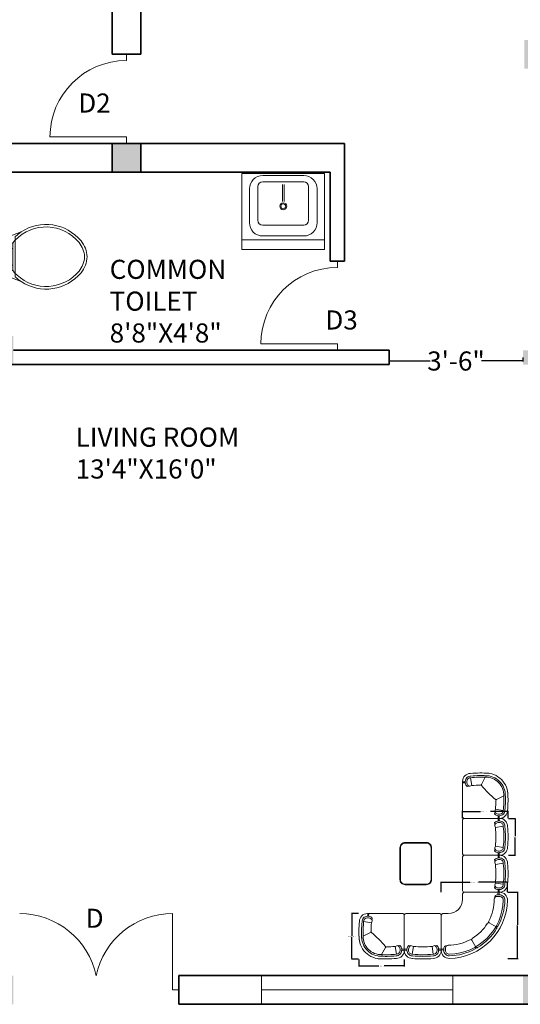
# Model space of a CAD drawing. Units: inches. Extents: x -36302355 to 648, y -221479757 to 75.
# Tile 13 of 37: x 285 to 442, y -580 to -271. Entities that reach past the tile are written whole.
import ezdxf

# ---------------------------------------------------------------- set-up
doc = ezdxf.new("R2010")
doc.units = ezdxf.units.IN
doc.header["$MEASUREMENT"] = 0
for name, color, linetype, lineweight in [('A-ANNO-DIMS', 2, 'Continuous', 18), ('A-ANNO-IDEN', 7, 'Continuous', 18), ('A-AREA-IDEN', 7, 'Continuous', 18), ('A-COLS', 7, 'Continuous', 35), ('A-COLS-PATT', 242, 'Continuous', 13), ('A-DOOR', 4, 'Continuous', 18), ('A-FLOR-FIXT', 9, 'Continuous', 18), ('A-FURN', 8, 'Continuous', 13), ('A-GLAZ', 142, 'Continuous', 18), ('A-WALL', 7, 'Continuous', 35)]:
    doc.layers.add(name, color=color, linetype=linetype, lineweight=lineweight)
doc.styles.get("Standard").update_dxf_attribs({"font": 'arial.ttf'})
doc.dimstyles.get("Standard").update_dxf_attribs({"dimtxt": 0.18, "dimasz": 0.18, "dimexe": 0.18, "dimexo": 0.0625, "dimgap": 0.09, "dimtad": 0, "dimtih": 1, "dimtoh": 1, "dimdec": 0, "dimzin": 0, "dimdsep": 46, "dimlunit": 3, "dimtxsty": 'Standard', "dimcen": 0.09, "dimadec": 0, "dimazin": 0, "dimtfac": 1, "dimtdec": 0, "dimtofl": 0, "dimtmove": 0, "dimatfit": 3, "dimfxl": 1, "dimtolj": 1, "dimtzin": 0, "dimarcsym": 0})

# ---------------------------------------------------------------- blocks, each defined once
blk = doc.blocks.new('*D5')
at = {"layer": 'A-ANNO-DIMS', "color": 0, "lineweight": -2, "transparency": 16777216}
for p, q in [((401.2, -376.83), (401.2, -378.08)), ((443.2, -376.83), (443.2, -378.08)), ((401.38, -377.9), (414.13, -377.9)), ((443.02, -377.9), (430.26, -377.9))]:
    blk.add_line(p, q, dxfattribs=at)
at = {"layer": 'A-ANNO-DIMS', "color": 0, "transparency": 16777216}
for points in [[(401.38, -377.87), (401.38, -377.93), (401.2, -377.9)], [(443.02, -377.87), (443.02, -377.93), (443.2, -377.9)]]:
    blk.add_solid(points, dxfattribs=at)
at = {"layer": 'Defpoints', "color": 0, "transparency": 16777216}
for p in [(401.2, -376.77), (443.2, -376.77), (443.2, -377.9)]:
    blk.add_point(p, dxfattribs=at)
at = {"layer": 'A-ANNO-DIMS', "color": 0, "transparency": 16777216, "insert": (422.2, -377.9), "char_height": 6, "attachment_point": 5}
blk.add_mtext('\\A1;3\'-6"', dxfattribs=at)
blk = doc.blocks.new('A$C707258B2')
at = {"color": 0}
for p, q in [((0.404, 0.342), (1.074, 0.342)), ((0.404, 0.292), (0.454, 0.292)), ((0.404, 0.262), (0.454, 0.262)), ((1.104, 0.312), (1.104, 0.212)), ((1.479, -0.063), (1.379, -0.063)), ((1.509, -0.763), (1.509, -0.093)), ((0.6, -0.238), (0.47, -0.313)), ((0.929, -0.567), (0.854, -0.697)), ((1.429, -0.763), (1.429, -0.713)), ((1.459, -0.763), (1.459, -0.712))]:
    blk.add_line(p, q, dxfattribs=at)
for centre, radius, start, end in [((0.404, 0.192), 0.15, 90, 181.1754), ((1.379, 0.212), 1.125, 181.1754, 268.8246), ((0.404, 0.192), 0.1, 90, 181.1754), ((1.379, 0.212), 1.075, 181.1754, 208.6357), ((0.404, 0.192), 0.07, 90, 181.1754), ((1.379, 0.212), 1.045, 181.1754, 268.8246), ((0.378, 0.317), 0.0362, 316.3972, 43.6028), ((0.368, 0.317), 0.0662, 337.8298, 22.1702), ((0.455, 0.256), 0.0357, 345.4262, 90.5555), ((0.454, 0.212), 0.05, 360, 90), ((1.379, 0.212), 0.875, 180, 208.4082), ((1.074, 0.312), 0.03, 360, 90), ((1.379, 0.212), 0.275, 180, 270), ((1.479, -0.093), 0.03, 360, 90), ((0.457, -0.291), 0.025, 208.6357, 300), ((0.482, -0.334), 0.025, 120, 211.3643), ((1.379, 0.212), 1.075, 211.3643, 238.6357), ((0.587, -0.216), 0.025, 300, 28.4082), ((0.612, -0.259), 0.025, 31.5918, 120), ((1.379, 0.212), 0.875, 211.5918, 238.4082), ((0.907, -0.555), 0.025, 330, 58.4082), ((0.951, -0.58), 0.025, 61.5918, 150), ((1.379, 0.212), 0.875, 241.5918, 270), ((0.832, -0.685), 0.025, 238.6357, 330), ((0.876, -0.71), 0.025, 150, 241.3643), ((1.379, 0.212), 1.075, 241.3643, 268.8246), ((1.379, -0.713), 0.05, 360, 90), ((1.425, -0.709), 0.0336, 354.6301, 109.3883), ((1.484, -0.799), 0.0662, 67.8298, 112.1702), ((1.359, -0.763), 0.15, 268.8246, 360), ((1.359, -0.763), 0.1, 268.8246, 360), ((1.359, -0.763), 0.07, 268.8246, 360), ((1.484, -0.789), 0.0362, 46.3972, 133.6028)]:
    blk.add_arc(centre, radius, start, end, dxfattribs=at)
blk = doc.blocks.new('part 01')
at = {"color": 0}
for p, q in [((-670, 700), (0, 700)), ((-591, 527), (-579, 561)), ((30, 30), (30, 670)), ((-591, 527), (-740, 550)), ((-591, 173), (-740, 150)), ((-670, 0), (0, 0)), ((-591, 173), (-579, 139))]:
    blk.add_line(p, q, dxfattribs=at)
for centre, radius, start, end in [((-670, 550), 150, 90, 181.1754), ((-670, 550), 100, 90, 181.1754), ((-670, 550), 70, 90, 181.1754), ((-660, 518), 133, 56.0897, 95.6132), ((-696, 675), 36.2, 316.3972, 43.6028), ((-660, 518), 103, 42.0066, 95.6132), ((-706, 675), 66.2, 337.8298, 22.1702), ((-600, 607), 25, 332.9608, 56.0897), ((-625, 620), 53.2, 321.0017, 332.9608), ((-602, 570), 25, 340, 42.0066), ((0, 670), 30, 0, 90), ((1178, 350), 2008, 174.2835, 185.7165), ((1178, 350), 1958, 174.2835, 185.7165), ((1178, 350), 1928, 174.2835, 185.7165), ((1178, 350), 1778, 174.2835, 185.7165), ((-670, 150), 150, 178.8246, 270), ((-670, 150), 100, 178.8246, 270), ((-670, 150), 70, 178.8246, 270), ((-660, 182), 133, 264.3868, 303.9103), ((-660, 182), 103, 264.3868, 317.9934), ((-696, 25), 36.2, 316.3972, 43.6028), ((-706, 25), 66.2, 337.8298, 22.1702), ((-600, 93), 25, 303.9103, 27.0392), ((-602, 130), 25, 317.9934, 20), ((-625, 80), 53.2, 27.0392, 38.9983), ((0, 30), 30, 270, 0)]:
    blk.add_arc(centre, radius, start, end, dxfattribs=at)
blk = doc.blocks.new('part02')
at = {"color": 0}
for p, q in [((0, -670), (0, 0)), ((30, 30), (700, 30)), ((621, -143), (609, -109)), ((621, -143), (770, -120)), ((640, -326), (778, -399)), ((173, -591), (139, -579)), ((173, -591), (150, -740)), ((356, -610), (429, -748))]:
    blk.add_line(p, q, dxfattribs=at)
for centre, radius, start, end in [((30, 0), 30, 90, 180), ((726, 5), 56.2, 153.6122, 206.6666), ((726, 5), 36.2, 136.3972, 223.6028), ((700, -120), 150, 0, 90), ((630, -63), 25, 123.9103, 207.0392), ((655, -50), 53.2, 207.0392, 218.9983), ((632, -100), 25, 137.9934, 200), ((690, -152), 103, 84.3868, 137.9934), ((689, -151), 132, 85.4378, 123.9887), ((-1148, -320), 1778, 0.3836, 5.7165), ((700, -121), 101, 357.5006, 89.858), ((700, -120), 70, 0, 90), ((-1228, -320), 2008, 357.7349, 5.7032), ((-1148, -320), 1958, 355.8657, 5.7165), ((-1148, -320), 2008, 355.818, 5.7165), ((2220, -2190), 2454, 130.6961, 139.3039), ((632, -344), 20, 62, 130.6961), ((650, -308), 20, 180.3836, 242), ((439, -409), 419, 268.2181, 1.7819), ((439, -409), 369, 268.2181, 1.7819), ((439, -409), 339, 268.2181, 1.7819), ((25, -696), 56.2, 63.3334, 116.3878), ((25, -696), 36.2, 46.3972, 133.6028), ((150, -670), 150, 180, 271.1754), ((182, -660), 133, 146.0897, 185.6132), ((150, -670), 100, 180, 271.1754), ((93, -600), 25, 62.9608, 146.0897), ((182, -660), 103, 132.0066, 185.6132), ((150, -670), 70, 180, 270), ((80, -625), 53.2, 51.0017, 62.9608), ((130, -602), 25, 70, 132.0066), ((350, 1258), 2008, 264.2968, 272.2651), ((350, 1178), 1778, 264.2835, 269.6164), ((338, -620), 20, 28, 89.6164), ((374, -602), 20, 139.3039, 208), ((350, 1178), 2008, 264.2835, 274.182), ((350, 1178), 1958, 264.2835, 274.1343)]:
    blk.add_arc(centre, radius, start, end, dxfattribs=at)
blk = doc.blocks.new('М14 600х655')
for p, q in [((-655, 600), (-655, 0)), ((-655, 600), (-655, 0)), ((-655, 0), (-655, 600)), ((0, 600), (-655, 600)), ((0, 0), (0, 600)), ((0, 525), (-655, 525)), ((-165.1, 494.1), (-489.9, 494.1)), ((-165.4, 408.4), (-490.2, 408.4)), ((-595.8, 388.1), (-595.8, 121.3)), ((-528.4, 370.1), (-528.4, 103.3)), ((-127.2, 103.3), (-127.2, 370.1)), ((-59.2, 121.3), (-59.2, 388.1)), ((-333.5, 87.1), (-333.5, 219.6)), ((-321.5, 87.1), (-321.5, 219.6)), ((-655, 0), (-655, 0)), ((-655, 0), (-655, 0)), ((-655, 0), (0, 0)), ((-655, 0), (0, 0)), ((-490.2, 65.1), (-165.4, 65.1)), ((-489.9, 15.4), (-165.1, 15.4))]:
    blk.add_line(p, q)
for radius in [27.6, 19.3]:
    blk.add_circle((-327.5, 258.9), radius)
for centre, radius, start, end in [((-489.9, 388.1), 105.9, 90, 180), ((-165.1, 388.1), 105.9, 0, 90), ((-490.2, 370.1), 38.2, 90, 180), ((-165.4, 370.1), 38.2, 0, 90), ((-489.9, 121.3), 105.9, 180, 270), ((-490.2, 103.3), 38.2, 180, 270), ((-165.4, 103.3), 38.2, 270, 0), ((-165.1, 121.3), 105.9, 270, 0)]:
    blk.add_arc(centre, radius, start, end)
blk = doc.blocks.new('WC-FLOOR-MOUNT')
for p, q in [((4.02, 15.38), (4.02, 16.49)), ((4.02, 15.38), (4.02, 10.15)), ((4.02, 4.92), (4.02, 10.15)), ((4.02, 3.8), (4.02, 4.92))]:
    blk.add_line(p, q)
for points in [[(4.02, 15.38, -0.448546), (24.05, 14.64, -0.162618), (25.78, 10.15, -0.470877)], [(5.85, 17.93, -0.383919), (24.66, 15.14, -0.163732), (26.58, 10.15, -0.359733)], [(0, 10.15), (0, 15.22, -0.31031), (0.43, 15.85), (5.85, 17.93, -0.209071)], [(4.02, 16.49, -0.040937), (5.85, 17.93, -0.163732)], [(3.22, 14.46), (2.11, 14.46, 1), (2.11, 12.77), (2.69, 12.77)], [(3.22, 14.46, -0.022712), (4.02, 15.38, -0.162618)], [(3.22, 10.15), (3.22, 14.46, -0.476108)], [(0, 10.15), (0, 5.07, 0.31031), (0.43, 4.45), (5.85, 2.37, 0.209071)], [(3.22, 10.15), (3.22, 5.84, 0.022712)], [(4.57, 4.39, 0.431639), (24.05, 5.66, 0.162618), (25.78, 10.15, 0.470877)], [(5.85, 2.37, 0.383919), (24.66, 5.15, 0.163732), (26.58, 10.15, 0.359733)], [(3.22, 5.84), (2.11, 5.84, -1), (2.11, 7.53), (2.69, 7.53)], [(3.22, 5.84, 0.022712), (4.02, 4.92, 0.162618)], [(4.02, 4.92, 0.014165), (4.57, 4.39, 0.162618)], [(4.02, 3.8, 0.040937), (5.85, 2.37, 0.163732)]]:
    blk.add_lwpolyline(points, format="xyb")
for points in [[(2.69, 12.77), (2.69, 7.53)], [(2.69, 12.77), (3.22, 12.77)], [(2.69, 7.53), (3.22, 7.53)]]:
    blk.add_lwpolyline(points)
blk = doc.blocks.new('WIN-60')
for p, q in [((60, 9), (0, 9)), ((0, 9), (0, 0)), ((60, 0), (60, 9)), ((0, 4.5), (60, 4.5)), ((0, 0), (60, 0))]:
    blk.add_line(p, q)
blk = doc.blocks.new('DOOR-SWING-24')
for p, q in [((0, 26), (0, 28)), ((0, 0), (0, 2)), ((0, 2), (24, 2))]:
    blk.add_line(p, q)
blk.add_arc((0, 2), 24, 0, 90)
blk = doc.blocks.new('*D35')
at = {"layer": 'A-ANNO-DIMS', "color": 0, "lineweight": -2, "transparency": 16777216}
for p, q in [((424.29, -521.53), (424.29, -519.27)), ((424.47, -519.45), (429.85, -519.45)), ((438.42, -519.45), (433.03, -519.45)), ((438.6, -521.53), (438.6, -519.27))]:
    blk.add_line(p, q, dxfattribs=at)
at = {"layer": 'A-ANNO-DIMS', "color": 0, "transparency": 16777216}
for points in [[(424.47, -519.42), (424.47, -519.48), (424.29, -519.45)], [(438.42, -519.42), (438.42, -519.48), (438.6, -519.45)]]:
    blk.add_solid(points, dxfattribs=at)
at = {"layer": 'Defpoints', "color": 0, "transparency": 16777216}
for p in [(424.29, -519.45), (424.29, -521.59), (438.6, -521.59)]:
    blk.add_point(p, dxfattribs=at)
at = {"layer": 'A-ANNO-DIMS', "color": 0, "transparency": 16777216, "insert": (431.44, -519.45), "char_height": 0.18, "attachment_point": 5}
blk.add_mtext('\\A1;SOFA SEAT 1\'-2 1/2" TYP.', dxfattribs=at)
blk = doc.blocks.new('*D36')
at = {"layer": 'A-ANNO-DIMS', "color": 0, "lineweight": -2, "transparency": 16777216}
for p, q in [((438.66, -521.59), (440.92, -521.59)), ((440.74, -521.77), (440.74, -527.21)), ((440.74, -533.02), (440.74, -527.58)), ((438.66, -533.2), (440.92, -533.2))]:
    blk.add_line(p, q, dxfattribs=at)
at = {"layer": 'A-ANNO-DIMS', "color": 0, "transparency": 16777216}
for points in [[(440.71, -521.77), (440.77, -521.77), (440.74, -521.59)], [(440.71, -533.02), (440.77, -533.02), (440.74, -533.2)]]:
    blk.add_solid(points, dxfattribs=at)
at = {"layer": 'Defpoints', "color": 0, "transparency": 16777216}
for p in [(438.6, -521.59), (440.74, -521.59), (438.6, -533.2)]:
    blk.add_point(p, dxfattribs=at)
at = {"layer": 'A-ANNO-DIMS', "color": 0, "transparency": 16777216, "insert": (440.74, -527.4), "char_height": 0.18, "attachment_point": 5}
blk.add_mtext('\\A1;0\'-11 1/2" TYP.', dxfattribs=at)
blk = doc.blocks.new('*D51')
at = {"layer": 'A-ANNO-DIMS', "color": 0, "lineweight": -2, "transparency": 16777216}
for p, q in [((391.6, -551.52), (389.34, -551.52)), ((389.52, -551.7), (389.52, -558.49)), ((389.52, -565.64), (389.52, -558.85)), ((391.6, -565.82), (389.34, -565.82))]:
    blk.add_line(p, q, dxfattribs=at)
at = {"layer": 'A-ANNO-DIMS', "color": 0, "transparency": 16777216}
for points in [[(389.49, -551.7), (389.55, -551.7), (389.52, -551.52)], [(389.49, -565.64), (389.55, -565.64), (389.52, -565.82)]]:
    blk.add_solid(points, dxfattribs=at)
at = {"layer": 'Defpoints', "color": 0, "transparency": 16777216}
for p in [(389.52, -551.52), (391.66, -551.52), (391.66, -565.82)]:
    blk.add_point(p, dxfattribs=at)
at = {"layer": 'A-ANNO-DIMS', "color": 0, "transparency": 16777216, "insert": (389.52, -558.67), "char_height": 0.18, "attachment_point": 5}
blk.add_mtext('\\A1;SOFA END 1\'-2 1/2" TYP.', dxfattribs=at)
blk = doc.blocks.new('*D52')
at = {"layer": 'A-ANNO-DIMS', "color": 0, "lineweight": -2, "transparency": 16777216}
for p, q in [((391.66, -565.89), (391.66, -568.15)), ((405.97, -565.89), (405.97, -568.15)), ((391.84, -567.97), (397.98, -567.97)), ((405.79, -567.97), (399.66, -567.97))]:
    blk.add_line(p, q, dxfattribs=at)
at = {"layer": 'A-ANNO-DIMS', "color": 0, "transparency": 16777216}
for points in [[(391.84, -567.94), (391.84, -568), (391.66, -567.97)], [(405.79, -567.94), (405.79, -568), (405.97, -567.97)]]:
    blk.add_solid(points, dxfattribs=at)
at = {"layer": 'Defpoints', "color": 0, "transparency": 16777216}
for p in [(391.66, -565.82), (405.97, -565.82), (391.66, -567.97)]:
    blk.add_point(p, dxfattribs=at)
at = {"layer": 'A-ANNO-DIMS', "color": 0, "transparency": 16777216, "insert": (398.82, -567.97), "char_height": 0.18, "attachment_point": 5}
blk.add_mtext('\\A1;1\'-2 1/2" TYP.', dxfattribs=at)
blk = doc.blocks.new('*D55')
at = {"layer": 'A-ANNO-DIMS', "color": 0, "lineweight": -2, "transparency": 16777216}
for p, q in [((417.57, -544.74), (417.57, -541.5)), ((417.75, -541.68), (426.7, -541.68)), ((438.21, -541.68), (429.27, -541.68)), ((438.39, -544.74), (438.39, -541.5))]:
    blk.add_line(p, q, dxfattribs=at)
at = {"layer": 'A-ANNO-DIMS', "color": 0, "transparency": 16777216}
for points in [[(417.75, -541.65), (417.75, -541.71), (417.57, -541.68)], [(438.21, -541.65), (438.21, -541.71), (438.39, -541.68)]]:
    blk.add_solid(points, dxfattribs=at)
at = {"layer": 'Defpoints', "color": 0, "transparency": 16777216}
for p in [(417.57, -541.68), (417.57, -544.8), (438.39, -544.8)]:
    blk.add_point(p, dxfattribs=at)
at = {"layer": 'A-ANNO-DIMS', "color": 0, "transparency": 16777216, "insert": (427.98, -541.68), "char_height": 0.18, "attachment_point": 5}
blk.add_mtext('\\A1;SOFA CORNER 1\'-9"', dxfattribs=at)
blk = doc.blocks.new('*D56')
at = {"layer": 'A-ANNO-DIMS', "color": 0, "lineweight": -2, "transparency": 16777216}
for p, q in [((438.45, -544.8), (441.69, -544.8)), ((441.51, -544.98), (441.51, -555.03)), ((441.51, -565.44), (441.51, -555.39)), ((438.45, -565.62), (441.69, -565.62))]:
    blk.add_line(p, q, dxfattribs=at)
at = {"layer": 'A-ANNO-DIMS', "color": 0, "transparency": 16777216}
for points in [[(441.48, -544.98), (441.54, -544.98), (441.51, -544.8)], [(441.48, -565.44), (441.54, -565.44), (441.51, -565.62)]]:
    blk.add_solid(points, dxfattribs=at)
at = {"layer": 'Defpoints', "color": 0, "transparency": 16777216}
for p in [(438.39, -544.8), (441.51, -544.8), (438.39, -565.62)]:
    blk.add_point(p, dxfattribs=at)
at = {"layer": 'A-ANNO-DIMS', "color": 0, "transparency": 16777216, "insert": (441.51, -555.21), "char_height": 0.18, "attachment_point": 5}
blk.add_mtext('\\A1;1\'-9"', dxfattribs=at)

msp = doc.modelspace()

# ---------------------------------------------------------------- hatches: boundary and pattern name
at = {"layer": 'A-COLS-PATT'}
h = msp.add_hatch(color=256, dxfattribs=at)
h.dxf.hatch_style = 1
h.paths.add_polyline_path([(145.2, 24.98), (145.2, 15.98), (154.2, 15.98), (154.2, 24.98)])
h.paths.add_polyline_path([(247.2, 15.98), (247.2, 24.98), (238.2, 24.98), (238.2, 15.98)])
h.paths.add_polyline_path([(387.64, 15.98), (395.7, 15.98), (395.7, 24.98), (387.64, 24.98)])
h.paths.add_polyline_path([(451.26, 24.98), (443.7, 24.98), (443.7, 15.98), (451.26, 15.98)])
h.paths.add_polyline_path([(596.2, 15.98), (605.2, 15.98), (605.2, 24.98), (596.2, 24.98)])
h.paths.add_polyline_path([(238.2, -122.02), (238.2, -131.02), (247.2, -131.02), (247.2, -122.02)])
h.paths.add_polyline_path([(395.7, -122.02), (387.46, -122.02), (387.46, -131.02), (395.7, -131.02)])
h.paths.add_polyline_path([(448.2, -131.02), (453.73, -131.02), (453.73, -122.02), (443.7, -122.02), (443.7, -131.02)])
h.paths.add_polyline_path([(596.2, -131.02), (605.2, -131.02), (605.2, -122.02), (596.2, -122.02)])
h.paths.add_polyline_path([(145.2, -176.97), (154.2, -176.97), (154.2, -167.02), (145.2, -167.02)])
h.paths.add_polyline_path([(314.2, -176.97), (323.2, -176.97), (323.2, -167.02), (314.2, -167.02)])
h.paths.add_polyline_path([(154.2, -314.02), (154.2, -309.52), (145.2, -309.52), (145.2, -314.02)])
h.paths.add_polyline_path([(314.2, -309.52), (314.2, -318.52), (323.2, -318.52), (323.2, -309.52)])
h.paths.add_polyline_path([(448.2, -277.02), (443.7, -277.02), (443.7, -286.02), (448.2, -286.02)])
h.paths.add_polyline_path([(283.2, -370.02), (274.2, -370.02), (274.2, -379.02), (283.2, -379.02), (283.2, -374.52)])
h.paths.add_polyline_path([(154.2, -370.02), (145.2, -370.02), (145.2, -379.02), (154.2, -379.02)])
h.paths.add_polyline_path([(443.2, -374.52), (443.2, -379.02), (452.2, -379.02), (452.2, -374.52)])
h.paths.add_polyline_path([(145.2, -580.02), (154.2, -580.02), (154.2, -571.02), (145.2, -571.02)])
h.paths.add_polyline_path([(274.2, -571.02), (274.2, -580.02), (283.2, -580.02), (283.2, -571.02)])
h.paths.add_polyline_path([(443.2, -580.02), (452.2, -580.02), (452.2, -571.02), (443.2, -571.02)])

# ---------------------------------------------------------------- linework, layer by layer
at = {"layer": 'A-COLS'}
for p, q in [((314.2, -309.52), (314.2, -318.52)), ((323.2, -309.52), (323.2, -318.52))]:
    msp.add_line(p, q, dxfattribs=at)
at = {"layer": 'A-DOOR'}
for q in [(333.2, -551.52), (335.2, -575.52)]:
    msp.add_line((333.2, -575.52), q, dxfattribs=at)
for centre, start, end in [((285.2, -576.04), 11.8123, 90), ((333.2, -576.04), 90, 168.1877)]:
    msp.add_arc(centre, 24.52, start, end, dxfattribs=at)
at = {"layer": 'A-FURN', "ltscale": 0.03}
for points in [[(412.89, -529.18), (406.25, -529.18, 0.414214), (404.6, -530.83), (404.6, -540.78, 0.414214), (406.25, -542.44), (412.89, -542.44, 0.414214), (414.54, -540.78), (414.54, -530.83, 0.414214)], [(412.89, -529.34), (406.25, -529.34, 0.414214), (404.76, -530.83), (404.76, -540.78, 0.414214), (406.25, -542.27), (412.89, -542.27, 0.414214), (414.38, -540.78), (414.38, -530.83, 0.414214)]]:
    msp.add_lwpolyline(points, format="xyb", close=True, dxfattribs=at)
at = {"layer": 'A-WALL'}
for p, q in [((314.2, -167.02), (314.2, -281.52)), ((323.2, -167.02), (323.2, -281.52)), ((318.7, -281.52), (314.2, -281.52)), ((318.7, -281.52), (323.2, -281.52)), ((274.2, -309.52), (387.2, -309.52)), ((387.2, -309.52), (387.2, -346.52)), ((278.7, -318.52), (382.7, -318.52)), ((382.7, -318.52), (382.7, -346.52)), ((384.95, -346.52), (382.7, -346.52)), ((384.95, -346.52), (387.2, -346.52)), ((283.2, -374.52), (401.2, -374.52)), ((401.2, -374.52), (401.2, -379.02)), ((145.2, -379.02), (314.2, -379.02)), ((314.2, -379.02), (401.2, -379.02)), ((335.2, -575.52), (335.2, -571.02)), ((335.2, -571.02), (605.2, -571.02)), ((335.2, -575.52), (335.2, -580.02)), ((335.2, -580.02), (605.2, -580.02))]:
    msp.add_line(p, q, dxfattribs=at)

# ---------------------------------------------------------------- block references
at = {"layer": 'A-DOOR', "extrusion": (0, 0, -1), "zscale": -1}
for p in [(-318.7, -309.52), (-384.95, -374.52)]:
    msp.add_blockref('DOOR-SWING-24', p, dxfattribs=at)
at = {"layer": 'A-FLOR-FIXT', "xscale": -0.0396455158158922, "yscale": 0.0396455158158922, "zscale": 0.0396455158158922, "rotation": 180}
msp.add_blockref('М14 600х655', (380.95, -319.03), dxfattribs=at)
at = {"layer": 'A-FLOR-FIXT'}
msp.add_blockref('WC-FLOOR-MOUNT', (279.79, -355.3), dxfattribs=at)
at = {"layer": 'A-FURN', "ltscale": 0.03}
for name, p, xscale, yscale, zscale, rotation in [('part02', (424.79, -521.59), 0.0165786247194503, 0.0165786247194503, 0.0165786247194503, 90.00000000000314), ('A$C707258B2', (423.24, -569.82), 16.57862471945027, 16.57862471945027, 16.57862471945027, 90.00000000000321), ('part 01', (405.97, -552.02), -0.0165786247194503, 0.0165786247194503, 0.0165786247194503, 270)]:
    msp.add_blockref(name, p, dxfattribs=dict(at, xscale=xscale, yscale=yscale, zscale=zscale, rotation=rotation))
at = {"layer": 'A-FURN', "ltscale": 0.03, "xscale": -0.0165786247194503, "yscale": 0.0165786247194503, "zscale": 0.0165786247194503}
for name, p in [('part 01', (424.79, -533.2)), ('part 01', (424.79, -544.8)), ('part02', (405.97, -552.02))]:
    msp.add_blockref(name, p, dxfattribs=at)
at = {"layer": 'A-GLAZ'}
msp.add_blockref('WIN-60', (361.17, -580.02), dxfattribs=at)

# ---------------------------------------------------------------- texts
at = {"layer": 'A-ANNO-IDEN', "char_height": 6, "attachment_point": 1}
for s, insert in [('D2', (303.59, -293.85)), ('D3', (381.18, -362.01)), ('D', (305.92, -549.99))]:
    msp.add_mtext(s, dxfattribs=dict(at, insert=insert))
at = {"layer": 'A-AREA-IDEN', "char_height": 6, "attachment_point": 1}
for s, insert in [('COMMON\\PTOILET\\P8\'8"X4\'8"', (313.45, -346.1)), ('LIVING ROOM\\P13\'4"X16\'0"', (302.78, -398.83))]:
    msp.add_mtext(s, dxfattribs=dict(at, insert=insert))

# ---------------------------------------------------------------- dimensions: what is measured, and where the dimension line sits
at = {"layer": 'A-ANNO-DIMS'}
dim = msp.add_linear_dim(base=(443.2, -377.9), p1=(401.2, -376.77), p2=(443.2, -376.77), dimstyle='Standard', override={"dimtxt": 6, "dimclrd": 0, "dimclre": 0, "dimclrt": 0}, dxfattribs=at)
dim.commit()
dim.dimension.update_dxf_attribs({"geometry": '*D5', "text_midpoint": (422.2, -377.9)})
for base, p1, p2, angle, text, picture, middle in [((424.29, -519.45), (438.6, -521.59), (424.29, -521.59), 180, 'SOFA SEAT <> TYP.', '*D35', (431.44, -519.45)), ((440.74, -521.59), (438.6, -533.2), (438.6, -521.59), 90, '<> TYP.', '*D36', (440.74, -527.4)), ((417.57, -541.68), (438.39, -544.8), (417.57, -544.8), 180, 'SOFA CORNER <>', '*D55', (427.98, -541.68)), ((389.52, -551.52), (391.66, -565.82), (391.66, -551.52), 90, 'SOFA END <> TYP.', '*D51', (389.52, -558.67)), ((391.66, -567.97), (405.97, -565.82), (391.66, -565.82), 180, '<> TYP.', '*D52', (398.82, -567.97))]:
    dim = msp.add_linear_dim(base=base, p1=p1, p2=p2, angle=angle, text=text, dimstyle='Standard', override={"dimdec": 1, "dimlfac": 1, "dimrnd": 0, "dimzin": 1, "dimdsep": 46, "dimlunit": 4, "dimfrac": 2}, dxfattribs=at)
    dim.commit()
    dim.dimension.update_dxf_attribs({"geometry": picture, "text_midpoint": middle})
dim = msp.add_linear_dim(base=(441.51, -544.8), p1=(438.39, -565.62), p2=(438.39, -544.8), angle=90, dimstyle='Standard', override={"dimdec": 1, "dimlfac": 1, "dimrnd": 0, "dimzin": 1, "dimdsep": 46, "dimlunit": 4, "dimfrac": 2}, dxfattribs=at)
dim.commit()
dim.dimension.update_dxf_attribs({"geometry": '*D56', "text_midpoint": (441.51, -555.21)})

doc.saveas('drawing.dxf')
